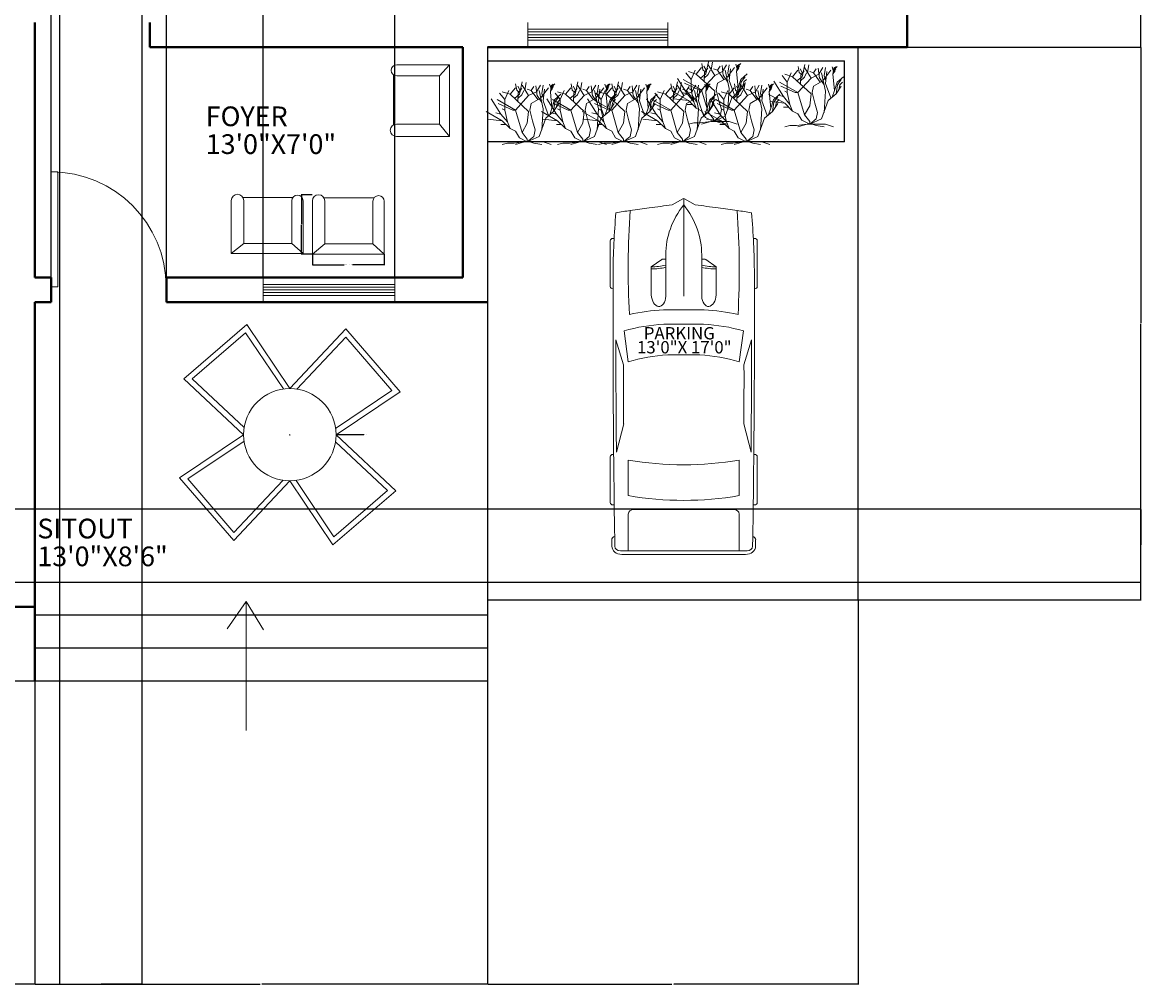
# Model space of a CAD drawing. Units: inches. Extents: x 12978 to 13669, y 46550 to 47327.
# Tile 2 of 5: x 13262 to 13669, y 46550 to 46901. Entities that reach past the tile are written whole.
import ezdxf

# ---------------------------------------------------------------- set-up
doc = ezdxf.new("R2010")
doc.units = ezdxf.units.IN
for name, color, linetype, lineweight in [('A-ANNO-DIMS', 2, 'Continuous', 18), ('A-ANNO-SYMB', 7, 'Continuous', 18), ('A-AREA-IDEN', 1, 'Continuous', 18), ('A-FLOR-OTLN', 7, 'Continuous', 25), ('C-PRKG-VEHI', 8, 'Continuous', 13), ('door', 4, 'Continuous', 20), ('furniture', 5, 'Continuous', 18), ('L-PLNT-TREE', 94, 'Continuous', 13), ('staircase', 7, 'Continuous', 25), ('wall', 7, 'Continuous', 40), ('window', 1, 'Continuous', 18)]:
    doc.layers.add(name, color=color, linetype=linetype, lineweight=lineweight)
doc.styles.get("Standard").update_dxf_attribs({"font": 'arial.ttf'})
doc.dimstyles.get("Standard").update_dxf_attribs({"dimtxt": 0.18, "dimasz": 0.18, "dimexe": 0.18, "dimexo": 0.0625, "dimgap": 0.09, "dimtad": 0, "dimtih": 1, "dimtoh": 1, "dimdec": 4, "dimzin": 0, "dimdsep": 46, "dimtxsty": 'Standard', "dimcen": 0.09, "dimadec": 0, "dimazin": 0, "dimtfac": 1, "dimtdec": 4, "dimtofl": 0, "dimtmove": 0, "dimatfit": 3, "dimfxl": 1, "dimtolj": 1, "dimtzin": 0, "dimarcsym": 0})

# ---------------------------------------------------------------- blocks, each defined once
blk = doc.blocks.new('*U2')
for p, q in [((0, 0), (0, -100)), ((750, 0), (750, -100))]:
    blk.add_line(p, q)
blk.add_lwpolyline([(0, 0), (0, 750), (43.75, 750), (43.75, 0)], close=True)
blk.add_arc((0, 0), 750, 0, 90)
blk = doc.blocks.new('*U6')
at = {"layer": 'furniture'}
for p, q in [((-20.08, -2.46), (0.34, 19.3)), ((0.34, 19.3), (20.08, -3.61)), ((-17.52, -2.66), (0.28, 16.31)), ((0.28, 16.31), (17.1, -3.21)), ((17.1, -3.21), (-3.41, -16.99)), ((20.08, -3.61), (-3.25, -19.3))]:
    blk.add_line(p, q, dxfattribs=at)
blk = doc.blocks.new('*U7')
at = {"layer": 'furniture', "transparency": 16777216}
for p, rotation in [((13339.66, 46770.42), 89.99999999999999), ((13338.88, 46731.04), 180), ((13378.26, 46730.25), 270)]:
    blk.add_blockref('*U6', p, dxfattribs=dict(at, rotation=rotation))
blk.add_blockref('*U6', (13379.05, 46769.63), dxfattribs=at)
blk = doc.blocks.new('*U11')
for p, q in [((21.1, 37.41), (21.1, 36.83)), ((46.55, 38.89), (22.35, 38.89)), ((47.8, 37.39), (47.8, 37.41)), ((87.99, 31.87), (74.76, 35.92)), ((134.31, 35.6), (119.29, 31.78)), ((135.45, 37.07), (135.45, 37.41)), ((136.7, 38.89), (160.9, 38.89)), ((162.15, 37.41), (162.15, 36.77)), ((70.03, 31.54), (86.41, 29.35)), ((186.47, -33.5), (186.47, 33.5)), ((188.4, -32.76), (188.4, 32.76)), ((138.42, 29.35), (157.25, 29.35)), ((164.52, 26.39), (164.52, -26.39)), ((186.47, 29.35), (167.01, 29.35)), ((32.27, 11.63), (36.13, 17.17)), ((36.13, 17.17), (50.94, 17.17)), ((3.27, 6.13), (0.1, 0.41)), ((29.77, 9.51), (51.68, 9.51)), ((32.12, 9.51), (32.12, 11.15)), ((58.92, -10.77), (58.92, 10.77)), ((66.55, -10.53), (66.55, 10.53)), ((82.74, 8.5), (82.74, -8.5)), ((186.47, -10.53), (186.47, 10.53)), ((0, 0), (51.68, 0)), ((0.1, -0.41), (3.27, -6.13)), ((29.77, -9.51), (51.68, -9.51)), ((32.12, -9.51), (32.12, -11.15)), ((32.27, -11.63), (36.13, -17.17)), ((36.13, -17.17), (50.94, -17.17)), ((86.41, -29.35), (70.03, -31.54)), ((157.25, -29.35), (138.42, -29.35)), ((167.01, -29.35), (186.47, -29.35)), ((87.99, -31.87), (74.76, -35.92)), ((134.31, -35.6), (119.29, -31.78)), ((21.1, -37.41), (21.1, -36.83)), ((46.55, -38.89), (22.35, -38.89)), ((47.8, -37.39), (47.8, -37.41)), ((135.45, -37.07), (135.45, -37.41)), ((136.7, -38.89), (160.9, -38.89)), ((162.15, -37.41), (162.15, -36.77))]:
    blk.add_line(p, q)
for centre, major_axis, ratio, start_param, end_param in [((266.03, -27.52), (0, 313.31), 0.842304, 1.367076, 1.39176), ((41.19, -490.86), (0, 528.23), 0.842304, 0.00281, 0.075598), ((22.35, 37.41), (0, -1.48), 0.842304, 3.141593, 4.712389), ((64.48, -10555.62), (0, 10593.03), 0.842304, -0.013397, 0.002797), ((46.55, 37.41), (0, 1.48), 0.842304, -1.570796, 0), ((64.48, -10555.62), (0, -10591.55), 0.842304, 3.133765, 3.140441), ((136.7, 37.41), (0, -1.48), 0.842304, 3.141593, 4.712389), ((160.9, 37.41), (0, 1.48), 0.842304, -1.570796, 0), ((180.63, 35.84), (0, 2.22), 0.842304, -0.013017, 1.249894), ((64.48, -10556.36), (0, 10595.31), 0.842304, -0.013397, -0.013017), ((183.98, 33.5), (0, -2.96), 0.842304, 1.570796, 3.128196), ((183.98, 32.76), (0, -5.25), 0.842304, 1.570796, 3.128196), ((37.47, -593.96), (0, -623.33), 0.842304, 3.096046, 3.200911), ((135.29, 5.39), (0, 81.77), 0.842304, 1.245306, 1.50788), ((95.79, -3666.35), (0, -3698.24), 0.842304, 3.134049, 3.144098), ((259.18, -27.52), (0, -305.3), 0.842304, 4.528606, 4.561838), ((134.4, 5.39), (0, -89.78), 0.842304, 4.449482, 4.652344), ((149.6, 2.8), (0, -79.58), 0.842304, 4.372215, 4.640744), ((17.08, 0), (0, 147.02), 0.842304, 4.511394, 4.913384), ((35.91, 0), (0, 147.02), 0.842304, 4.511394, 4.913384), ((167.01, 26.39), (0, 2.96), 0.842304, 0, 1.570796), ((-204.49, 52.4), (0, -250.96), 0.842304, 1.385369, 1.434372), ((13.04, 17.01), (0, 27.42), 0.842304, 4.435146, 4.718221), ((14.2, 17.01), (0, 27.42), 0.842304, 4.435146, 4.718221), ((50.79, 13.34), (6.34, -0.36), 0.603834, -1.395552, 1.581315), ((29.77, -46.66), (0, 56.17), 0.842304, 0, 0.590319), ((32.75, 11.15), (0, 0.74), 0.842304, 0.879714, 1.570796), ((0.62, 0), (0, -0.74), 0.842304, 4.131459, 5.293319), ((29.77, 46.66), (0, 56.17), 0.842304, 2.551274, 3.141593), ((-204.49, -52.4), (0, 250.96), 0.842304, -1.434372, -1.385369), ((32.75, -11.15), (0, -0.74), 0.842304, 4.712389, 5.403472), ((13.04, -17.01), (0, -27.42), 0.842304, 1.564964, 1.848039), ((14.2, -17.01), (0, -27.42), 0.842304, 1.564964, 1.848039), ((134.4, -5.39), (0, -89.78), 0.842304, -1.510751, -1.307889), ((135.29, -5.39), (0, -81.77), 0.842304, -1.50788, -1.245306), ((149.6, -2.8), (0, -79.58), 0.842304, -1.499151, -1.230623), ((259.18, 27.52), (0, 305.3), 0.842304, 1.721348, 1.754579), ((266.03, 27.52), (0, 313.31), 0.842304, 1.749832, 1.774517), ((37.47, 593.96), (0, -623.33), 0.842304, -0.059319, 0.045547), ((167.01, -26.39), (0, -2.96), 0.842304, 4.712389, 6.283185), ((95.79, 3666.35), (0, -3698.24), 0.842304, -0.002505, 0.007544), ((183.98, -33.5), (0, 2.96), 0.842304, 3.15499, 4.712389), ((183.98, -32.76), (0, -5.25), 0.842304, 0.013397, 1.570796), ((41.19, 490.86), (0, -528.23), 0.842304, -0.075598, -0.00281), ((22.35, -37.41), (0, 1.48), 0.842304, 1.570796, 3.141593), ((64.48, 10555.62), (0, 10593.03), 0.842304, 3.138796, 3.15499), ((46.55, -37.41), (0, -1.48), 0.842304, 0, 1.570796), ((64.48, 10555.62), (0, -10591.55), 0.842304, 0.001152, 0.007828), ((136.7, -37.41), (0, -1.48), 0.842304, -1.570796, 0), ((160.9, -37.41), (0, 1.48), 0.842304, 3.141593, 4.712389), ((180.63, -35.84), (0, -2.22), 0.842304, -1.249894, 0.013017), ((64.48, 10556.36), (0, 10595.31), 0.842304, 3.15461, 3.15499)]:
    blk.add_ellipse(centre, major_axis=major_axis, ratio=ratio, start_param=start_param, end_param=end_param)
at = {"extrusion": (0, 0, -1)}
blk.add_ellipse((50.79, -13.34), major_axis=(6.34, 0.36), ratio=0.603834, start_param=-1.395552, end_param=1.581315, dxfattribs=at)
blk = doc.blocks.new('*U13')
for p, q in [((-14.88, 18.24), (-12.96, 20.64)), ((-12.471, 19.775), (-12.898, 22.044)), ((-11.28, 19.619), (-12.104, 21.184)), ((-11.921, 18.836), (-10.64, 20.401)), ((-11.433, 18.289), (-10.457, 22.749)), ((-8.16, 17.76), (-10.56, 21.6)), ((-9.48, 19.775), (-8.992, 22.592)), ((-7.2, 19.68), (-6.24, 21.12)), ((-5.086, 17.741), (-5.513, 21.34)), ((-5.28, 19.2), (-3.84, 21.6)), ((-3.84, 16.8), (-0.96, 20.64)), ((-3.377, 18.602), (-2.888, 21.575)), ((-0.508, 21.888), (-0.081, 20.558)), ((-0.203, 19.149), (0.102, 21.34)), ((-0.142, 19.384), (0.59, 20.401)), ((-0.02, 20.01), (0.896, 21.105)), ((0.041, 20.714), (1.384, 22.044)), ((0.102, 21.34), (0.835, 21.888)), ((-18.24, 11.04), (-21.755, 16.655)), ((-12.96, 12.48), (-19.68, 16.32)), ((-16.8, 16.32), (-18.72, 18.72)), ((-14.88, 18.24), (-17.76, 19.2)), ((-16.8, 16.32), (-15.36, 19.68)), ((-16.8, 12.48), (-16.8, 16.32)), ((-8.16, 12), (-14.88, 18.24)), ((-13.325, 16.724), (-11.433, 18.289)), ((-12.96, 12.48), (-8.16, 17.76)), ((-11.677, 19.071), (-12.471, 19.775)), ((-12.043, 15.628), (-11.921, 18.836)), ((-11.982, 16.802), (-10.579, 18.054)), ((-10.579, 18.054), (-9.846, 19.697)), ((-7.2, 19.68), (-8.64, 20.16)), ((-8.16, 17.76), (-5.28, 19.2)), ((-4.8, 16.32), (-7.2, 19.68)), ((-7.2, 14.88), (-3.84, 16.8)), ((-3.377, 15.315), (-5.086, 17.819)), ((-2.88, 12.96), (-4.32, 19.68)), ((-2.766, 16.802), (-3.377, 18.602)), ((-2.88, 15.84), (-2.4, 20.16)), ((0.346, 13.203), (-0.203, 19.149)), ((1.323, 16.254), (3.642, 18.289)), ((1.44, 15.36), (2.88, 17.28)), ((2.4, 15.36), (3.36, 16.32)), ((-13.92, 12.48), (-19.2, 14.88)), ((-16.8, 12.48), (-17.76, 12.96)), ((-15.84, 8.16), (-16.8, 12.48)), ((-12.96, 12.48), (-13.92, 12.48)), ((-10.56, 4.32), (-12.96, 12.48)), ((-7.68, 12.48), (-7.2, 14.88)), ((-6.72, 8.64), (-7.68, 12.48)), ((-3.36, 5.28), (-2.88, 12.96)), ((-0.96, 10.56), (-2.88, 15.84)), ((-0.48, 10.8), (0.346, 13.203)), ((0.346, 13.203), (1.323, 16.254)), ((0.96, 12), (1.44, 15.36)), ((0.96, 12), (2.88, 14.88)), ((1.92, 13.44), (2.4, 15.36)), ((-17.76, 8.64), (-23.663, 11.961)), ((-17.76, 8.64), (-23.128, 9.222)), ((-18.24, 11.04), (-20.16, 11.52)), ((-15.84, 8.16), (-18.24, 11.04)), ((-14.88, 5.76), (-17.76, 8.64)), ((-14.88, 5.76), (-15.84, 8.16)), ((-8.64, 7.68), (-8.16, 12)), ((-5.76, 5.28), (-6.72, 8.64)), ((-4.32, 2.88), (-1.92, 9.6)), ((-1.92, 9.6), (0.96, 12)), ((-16.32, 7.2), (-18.24, 7.2)), ((-12.96, 4.8), (-14.88, 5.76)), ((-11.52, 2.4), (-12.96, 4.8)), ((-10.56, 4.32), (-8.64, 7.68)), ((-8.64, 1.92), (-10.56, 4.32)), ((-6.24, 2.88), (-5.76, 5.28)), ((-15.84, 0.48), (-17.76, 0)), ((-13.44, 0.48), (-15.84, 0.48)), ((-9.6, 0.96), (-13.44, 0.48)), ((-9.6, 0.96), (-12.96, 0)), ((-8.64, 0.96), (-11.52, 2.4)), ((-9.6, 0.96), (-7.68, 0.96)), ((-8.64, 0.96), (-4.32, 2.88)), ((-8.64, 0.96), (-6.24, 2.88)), ((-8.64, 0.96), (-8.64, 1.92)), ((-8.64, 0.96), (-2.88, 0.96)), ((-7.68, 0.96), (-6.24, 0.48)), ((-6.24, 0.48), (-3.36, 0)), ((-2.88, 0.96), (0, 0))]:
    blk.add_line(p, q)
blk = doc.blocks.new('WINDOW-51')
for p, q in [((0, 0), (0, 9)), ((51.08, 0), (51.08, 9)), ((0, 6.5), (51.08, 6.5)), ((0, 5.5), (51.08, 5.5)), ((0, 4.5), (51.08, 4.5)), ((0, 3.5), (51.08, 3.5)), ((0, 2.5), (51.08, 2.5))]:
    blk.add_line(p, q)
blk = doc.blocks.new('CHAIR-LOUNGE')
for p, q in [((21.6, 26.17), (2.34, 26.17)), ((17.92, 22.06), (21.6, 26.17)), ((21.6, 0), (21.6, 26.17)), ((1.14, 4.21), (1.14, 22.45)), ((2.34, 22.06), (17.92, 22.06)), ((17.92, 22.06), (17.92, 4.51)), ((17.92, 4.51), (2.25, 4.51)), ((17.92, 4.51), (21.6, 0)), ((2.25, 0), (21.6, 0))]:
    blk.add_line(p, q)
for centre, radius in [((2.34, 24.11), 2.05), ((2.25, 2.25), 2.25)]:
    blk.add_arc(centre, radius, 90, 270)
blk = doc.blocks.new('*D41')
at = {"layer": 'A-ANNO-DIMS', "color": 0, "lineweight": -2, "transparency": 16777216}
for p, q in [((13367.21, 46816.14), (13367.21, 46812.09)), ((13393.37, 46816.14), (13393.37, 46812.09)), ((13367.39, 46812.27), (13378.78, 46812.27)), ((13393.19, 46812.27), (13381.81, 46812.27))]:
    blk.add_line(p, q, dxfattribs=at)
at = {"layer": 'A-ANNO-DIMS', "color": 0, "transparency": 16777216}
for points in [[(13367.39, 46812.3), (13367.39, 46812.24), (13367.21, 46812.27)], [(13393.19, 46812.3), (13393.19, 46812.24), (13393.37, 46812.27)]]:
    blk.add_solid(points, dxfattribs=at)
at = {"layer": 'Defpoints', "color": 0, "transparency": 16777216}
for p in [(13367.21, 46816.2), (13393.37, 46816.2), (13393.37, 46812.27)]:
    blk.add_point(p, dxfattribs=at)
at = {"layer": 'A-ANNO-DIMS', "color": 0, "transparency": 16777216, "insert": (13380.29, 46812.27), "char_height": 0.18, "attachment_point": 5}
blk.add_mtext('\\A1;LOUNGE CHAIR 26 TYP.', dxfattribs=at)
blk = doc.blocks.new('*D42')
at = {"layer": 'A-ANNO-DIMS', "color": 0, "lineweight": -2, "transparency": 16777216}
for p, q in [((13367.15, 46837.79), (13363.1, 46837.79)), ((13363.28, 46837.61), (13363.28, 46827.18)), ((13363.28, 46816.38), (13363.28, 46826.82)), ((13367.15, 46816.2), (13363.1, 46816.2))]:
    blk.add_line(p, q, dxfattribs=at)
at = {"layer": 'A-ANNO-DIMS', "color": 0, "transparency": 16777216}
for points in [[(13363.25, 46837.61), (13363.31, 46837.61), (13363.28, 46837.79)], [(13363.25, 46816.38), (13363.31, 46816.38), (13363.28, 46816.2)]]:
    blk.add_solid(points, dxfattribs=at)
at = {"layer": 'Defpoints', "color": 0, "transparency": 16777216}
for p in [(13367.21, 46837.79), (13363.28, 46816.2), (13367.21, 46816.2)]:
    blk.add_point(p, dxfattribs=at)
at = {"layer": 'A-ANNO-DIMS', "color": 0, "transparency": 16777216, "insert": (13363.28, 46827), "char_height": 0.18, "attachment_point": 5}
blk.add_mtext('\\A1;22 TYP.', dxfattribs=at)
blk = doc.blocks.new('*D57')
at = {"layer": 'A-ANNO-DIMS', "color": 0, "lineweight": -2, "transparency": 16777216}
for p, q in [((13575.07, 47080.63), (13669.26, 47080.63)), ((13669.08, 47080.45), (13669.08, 46986.32)), ((13669.08, 46891.81), (13669.08, 46985.95)), ((13584.07, 46891.63), (13669.26, 46891.63))]:
    blk.add_line(p, q, dxfattribs=at)
at = {"layer": 'A-ANNO-DIMS', "color": 0, "transparency": 16777216}
for points in [[(13669.05, 47080.45), (13669.11, 47080.45), (13669.08, 47080.63)], [(13669.05, 46891.81), (13669.11, 46891.81), (13669.08, 46891.63)]]:
    blk.add_solid(points, dxfattribs=at)
at = {"layer": 'Defpoints', "color": 0, "transparency": 16777216}
for p in [(13575.01, 47080.63), (13669.08, 47080.63), (13584.01, 46891.63)]:
    blk.add_point(p, dxfattribs=at)
at = {"layer": 'A-ANNO-DIMS', "color": 0, "transparency": 16777216, "insert": (13669.08, 46986.13), "char_height": 0.18, "attachment_point": 5}
blk.add_mtext('\\A1;189', dxfattribs=at)
blk = doc.blocks.new('*D59')
at = {"layer": 'A-ANNO-DIMS', "color": 0, "lineweight": -2, "transparency": 16777216}
for p, q in [((13566.15, 46891.63), (13669.26, 46891.63)), ((13669.08, 46891.45), (13669.08, 46791.06)), ((13669.08, 46690.31), (13669.08, 46790.7)), ((13566.15, 46690.13), (13669.26, 46690.13))]:
    blk.add_line(p, q, dxfattribs=at)
at = {"layer": 'A-ANNO-DIMS', "color": 0, "transparency": 16777216}
for points in [[(13669.05, 46891.45), (13669.11, 46891.45), (13669.08, 46891.63)], [(13669.05, 46690.31), (13669.11, 46690.31), (13669.08, 46690.13)]]:
    blk.add_solid(points, dxfattribs=at)
at = {"layer": 'Defpoints', "color": 0, "transparency": 16777216}
for p in [(13566.09, 46891.63), (13669.08, 46891.63), (13566.09, 46690.13)]:
    blk.add_point(p, dxfattribs=at)
at = {"layer": 'A-ANNO-DIMS', "color": 0, "transparency": 16777216, "insert": (13669.08, 46790.88), "char_height": 0.18, "attachment_point": 5}
blk.add_mtext('\\A1;201.5', dxfattribs=at)
blk = doc.blocks.new('*D60')
at = {"layer": 'A-ANNO-DIMS', "color": 0, "lineweight": -2, "transparency": 16777216}
for p, q in [((13059.005025, 46660.571951), (13059.005025, 46549.877451)), ((13266.005025, 46660.571951), (13266.005025, 46549.877451)), ((13059.185025, 46550.057451), (13162.214643, 46550.057451)), ((13265.825025, 46550.057451), (13162.795407, 46550.057451))]:
    blk.add_line(p, q, dxfattribs=at)
at = {"layer": 'A-ANNO-DIMS', "color": 0, "transparency": 16777216}
for points in [[(13059.185025, 46550.087451), (13059.185025, 46550.027451), (13059.005025, 46550.057451)], [(13265.825025, 46550.087451), (13265.825025, 46550.027451), (13266.005025, 46550.057451)]]:
    blk.add_solid(points, dxfattribs=at)
at = {"layer": 'Defpoints', "color": 0, "transparency": 16777216}
for p in [(13059.005025, 46660.634451), (13266.005025, 46660.634451), (13266.005025, 46550.057451)]:
    blk.add_point(p, dxfattribs=at)
at = {"layer": 'A-ANNO-DIMS', "color": 0, "transparency": 16777216, "insert": (13162.505025, 46550.057451), "char_height": 0.18, "attachment_point": 5}
blk.add_mtext('\\A1;207', dxfattribs=at)
blk = doc.blocks.new('*D61')
at = {"layer": 'A-ANNO-DIMS', "color": 0, "lineweight": -2, "transparency": 16777216}
for p, q in [((13266.01, 46660.57), (13266.01, 46549.88)), ((13431.01, 46660.57), (13431.01, 46549.88)), ((13266.19, 46550.06), (13348.22, 46550.06)), ((13430.83, 46550.06), (13348.79, 46550.06))]:
    blk.add_line(p, q, dxfattribs=at)
at = {"layer": 'A-ANNO-DIMS', "color": 0, "transparency": 16777216}
for points in [[(13266.19, 46550.09), (13266.19, 46550.03), (13266.01, 46550.06)], [(13430.83, 46550.09), (13430.83, 46550.03), (13431.01, 46550.06)]]:
    blk.add_solid(points, dxfattribs=at)
at = {"layer": 'Defpoints', "color": 0, "transparency": 16777216}
for p in [(13266.01, 46660.63), (13431.01, 46660.63), (13431.01, 46550.06)]:
    blk.add_point(p, dxfattribs=at)
at = {"layer": 'A-ANNO-DIMS', "color": 0, "transparency": 16777216, "insert": (13348.51, 46550.06), "char_height": 0.18, "attachment_point": 5}
blk.add_mtext('\\A1;165', dxfattribs=at)
blk = doc.blocks.new('*D62')
at = {"layer": 'A-ANNO-DIMS', "color": 0, "lineweight": -2, "transparency": 16777216}
for p, q in [((13431.01, 46690.07), (13431.01, 46549.88)), ((13566.09, 46690.07), (13566.09, 46549.88)), ((13431.19, 46550.06), (13498.18, 46550.06)), ((13565.91, 46550.06), (13498.92, 46550.06))]:
    blk.add_line(p, q, dxfattribs=at)
at = {"layer": 'A-ANNO-DIMS', "color": 0, "transparency": 16777216}
for points in [[(13431.19, 46550.09), (13431.19, 46550.03), (13431.01, 46550.06)], [(13565.91, 46550.09), (13565.91, 46550.03), (13566.09, 46550.06)]]:
    blk.add_solid(points, dxfattribs=at)
at = {"layer": 'Defpoints', "color": 0, "transparency": 16777216}
for p in [(13431.01, 46690.13), (13566.09, 46690.13), (13566.09, 46550.06)]:
    blk.add_point(p, dxfattribs=at)
at = {"layer": 'A-ANNO-DIMS', "color": 0, "transparency": 16777216, "insert": (13498.55, 46550.06), "char_height": 0.18, "attachment_point": 5}
blk.add_mtext('\\A1;135.1', dxfattribs=at)
blk = doc.blocks.new('*D63')
at = {"layer": 'A-ANNO-DIMS', "color": 0, "lineweight": -2, "transparency": 16777216}
for p, q in [((13275.01, 47169.07), (13275.01, 46549.88)), ((13305.01, 47169.07), (13305.01, 46549.88)), ((13275.19, 46550.06), (13289.79, 46550.06)), ((13304.83, 46550.06), (13290.22, 46550.06))]:
    blk.add_line(p, q, dxfattribs=at)
at = {"layer": 'A-ANNO-DIMS', "color": 0, "transparency": 16777216}
for points in [[(13275.19, 46550.09), (13275.19, 46550.03), (13275.01, 46550.06)], [(13304.83, 46550.09), (13304.83, 46550.03), (13305.01, 46550.06)]]:
    blk.add_solid(points, dxfattribs=at)
at = {"layer": 'Defpoints', "color": 0, "transparency": 16777216}
for p in [(13275.01, 47169.13), (13305.01, 47169.13), (13305.01, 46550.06)]:
    blk.add_point(p, dxfattribs=at)
at = {"layer": 'A-ANNO-DIMS', "color": 0, "transparency": 16777216, "insert": (13290.01, 46550.06), "char_height": 0.18, "attachment_point": 5}
blk.add_mtext('\\A1;30', dxfattribs=at)
blk = doc.blocks.new('*D64')
at = {"layer": 'A-ANNO-DIMS', "color": 0, "lineweight": -2, "transparency": 16777216}
for p, q in [((13272.01, 46807.7), (13272.01, 47304.06)), ((13272.19, 47303.88), (13292.78, 47303.88)), ((13313.83, 47303.88), (13293.23, 47303.88)), ((13314.01, 46807.7), (13314.01, 47304.06))]:
    blk.add_line(p, q, dxfattribs=at)
at = {"layer": 'A-ANNO-DIMS', "color": 0, "transparency": 16777216}
for points in [[(13272.19, 47303.91), (13272.19, 47303.85), (13272.01, 47303.88)], [(13313.83, 47303.91), (13313.83, 47303.85), (13314.01, 47303.88)]]:
    blk.add_solid(points, dxfattribs=at)
at = {"layer": 'Defpoints', "color": 0, "transparency": 16777216}
for p in [(13314.01, 47303.88), (13272.01, 46807.63), (13314.01, 46807.63)]:
    blk.add_point(p, dxfattribs=at)
at = {"layer": 'A-ANNO-DIMS', "color": 0, "transparency": 16777216, "insert": (13293.01, 47303.88), "char_height": 0.18, "attachment_point": 5}
blk.add_mtext('\\A1;42', dxfattribs=at)
blk = doc.blocks.new('*D65')
at = {"layer": 'A-ANNO-DIMS', "color": 0, "lineweight": -2, "transparency": 16777216}
for p, q in [((13349.22, 46807.7), (13349.22, 47304.06)), ((13349.4, 47303.88), (13373, 47303.88)), ((13397.04, 47303.88), (13373.45, 47303.88)), ((13397.22, 46807.7), (13397.22, 47304.06))]:
    blk.add_line(p, q, dxfattribs=at)
at = {"layer": 'A-ANNO-DIMS', "color": 0, "transparency": 16777216}
for points in [[(13349.4, 47303.91), (13349.4, 47303.85), (13349.22, 47303.88)], [(13397.04, 47303.91), (13397.04, 47303.85), (13397.22, 47303.88)]]:
    blk.add_solid(points, dxfattribs=at)
at = {"layer": 'Defpoints', "color": 0, "transparency": 16777216}
for p in [(13397.22, 47303.88), (13349.22, 46807.63), (13397.22, 46807.63)]:
    blk.add_point(p, dxfattribs=at)
at = {"layer": 'A-ANNO-DIMS', "color": 0, "transparency": 16777216, "insert": (13373.22, 47303.88), "char_height": 0.18, "attachment_point": 5}
blk.add_mtext('\\A1;48', dxfattribs=at)
blk = doc.blocks.new('*D78')
at = {"layer": 'A-ANNO-DIMS', "color": 0, "lineweight": -2, "transparency": 16777216}
for p, q in [((13224.37, 46723.29), (13669.26, 46723.29)), ((13669.08, 46723.11), (13669.08, 46710.15)), ((13669.08, 46696.81), (13669.08, 46709.78)), ((13257.07, 46696.63), (13669.26, 46696.63))]:
    blk.add_line(p, q, dxfattribs=at)
at = {"layer": 'A-ANNO-DIMS', "color": 0, "transparency": 16777216}
for points in [[(13669.05, 46723.11), (13669.11, 46723.11), (13669.08, 46723.29)], [(13669.05, 46696.81), (13669.11, 46696.81), (13669.08, 46696.63)]]:
    blk.add_solid(points, dxfattribs=at)
at = {"layer": 'Defpoints', "color": 0, "transparency": 16777216}
for p in [(13224.3, 46723.29), (13669.08, 46723.29), (13257.01, 46696.63)]:
    blk.add_point(p, dxfattribs=at)
at = {"layer": 'A-ANNO-DIMS', "color": 0, "transparency": 16777216, "insert": (13669.08, 46709.96), "char_height": 0.18, "attachment_point": 5}
blk.add_mtext('\\A1;26.66', dxfattribs=at)
blk = doc.blocks.new('*D79')
at = {"layer": 'A-ANNO-DIMS', "color": 0, "lineweight": -2, "transparency": 16777216}
for p, q in [((13358.87, 46750.33), (13359.05, 46750.33)), ((13358.96, 46750.24), (13358.96, 46750.42)), ((13385.9, 46750.34), (13375.98, 46750.33))]:
    blk.add_line(p, q, dxfattribs=at)
at = {"layer": 'A-ANNO-DIMS', "color": 0, "transparency": 16777216}
blk.add_solid([(13375.98, 46750.37), (13375.98, 46750.31), (13375.8, 46750.33)], dxfattribs=at)
at = {"layer": 'Defpoints', "color": 0, "transparency": 16777216}
for p in [(13342.13, 46750.33), (13375.8, 46750.33)]:
    blk.add_point(p, dxfattribs=at)
at = {"layer": 'A-ANNO-DIMS', "color": 0, "transparency": 16777216, "insert": (13386.39, 46750.34), "char_height": 0.18, "attachment_point": 5}
blk.add_mtext('\\A1;∅33.67', dxfattribs=at)

msp = doc.modelspace()

# ---------------------------------------------------------------- linework, layer by layer
at = {"layer": 'A-ANNO-SYMB'}
for p, q in [((13343.0969, 46689.5271), (13336.0741, 46679.6103)), ((13343.0969, 46642.5353), (13343.0969, 46689.5271)), ((13343.0969, 46689.5271), (13349.3877, 46679.2043))]:
    msp.add_line(p, q, dxfattribs=at)
at = {"layer": 'A-FLOR-OTLN'}
for p, q in [((13431.005, 46891.6345), (13431.005, 46660.6345)), ((13566.0922, 46857.1263), (13566.0922, 46891.6345)), ((13431.005, 46886.6345), (13561.0922, 46886.6345)), ((13561.0922, 46857.1263), (13561.0922, 46886.6345)), ((13059.005, 46660.6345), (13431.005, 46660.6345))]:
    msp.add_line(p, q, dxfattribs=at)
msp.add_lwpolyline([(13561.0922, 46857.1263), (13431.005, 46857.1263), (13431.005, 46690.1305), (13566.0922, 46690.1305), (13566.0922, 46857.1263)], dxfattribs=at)
at = {"layer": 'furniture'}
msp.add_circle((13358.9612, 46750.3348), 16.8359, dxfattribs=at)
at = {"layer": 'staircase'}
for p, q in [((13266.005, 46696.6345), (13431.005, 46696.6345)), ((13266.005, 46684.6345), (13431.005, 46684.6345)), ((13266.005, 46672.6345), (13431.005, 46672.6345))]:
    msp.add_line(p, q, dxfattribs=at)
at = {"layer": 'wall'}
for p, q in [((13584.005, 47266.6345), (13584.005, 46891.6345)), ((13266.005, 46900.6345), (13266.005, 46807.6345)), ((13308.005, 46900.6345), (13308.005, 46891.6345)), ((13308.005, 46891.6345), (13422.005, 46891.6345)), ((13422.005, 46891.6345), (13422.005, 46807.6345)), ((13431.005, 46891.6345), (13584.005, 46891.6345)), ((13266.005, 46807.6345), (13272.005, 46807.6345)), ((13272.005, 46807.6345), (13272.005, 46798.6345)), ((13314.005, 46807.6345), (13314.005, 46798.6345)), ((13314.005, 46807.6345), (13422.005, 46807.6345)), ((13266.005, 46798.6345), (13272.005, 46798.6345)), ((13266.005, 46798.6345), (13266.005, 46660.6345)), ((13314.005, 46798.6345), (13431.005, 46798.6345)), ((13059.005, 46687.6345), (13266.005, 46687.6345))]:
    msp.add_line(p, q, dxfattribs=at)
at = {"layer": 'window'}
for p, q in [((13349.2243, 46798.6345), (13349.2243, 46807.6345)), ((13349.2243, 46805.1345), (13397.2243, 46805.1345)), ((13397.2243, 46798.6345), (13397.2243, 46807.6345)), ((13349.2243, 46804.1345), (13397.2243, 46804.1345)), ((13349.2243, 46803.1345), (13397.2243, 46803.1345)), ((13349.2243, 46802.1345), (13397.2243, 46802.1345)), ((13349.2243, 46801.1345), (13397.2243, 46801.1345))]:
    msp.add_line(p, q, dxfattribs=at)

# ---------------------------------------------------------------- block references
at = {"layer": 'C-PRKG-VEHI', "xscale": 0.6887919479552651, "yscale": 0.6887919479552651, "zscale": 0.6887919479552651, "rotation": 270}
msp.add_blockref('*U11', (13502.5212, 46836.4367), dxfattribs=at)
at = {"layer": 'door', "xscale": 0.0558759688399716, "yscale": 0.0558759688399716, "zscale": 0.0558759688399716}
msp.add_blockref('*U2', (13272.005, 46804.222), dxfattribs=at)
at = {"layer": 'furniture'}
for name, p in [('CHAIR-LOUNGE', (13395.5871, 46859.0438)), ('*U7', (0, 0))]:
    msp.add_blockref(name, p, dxfattribs=at)
for p, rotation in [((13337.649, 46837.9701), 269.9999999999682), ((13367.208, 46837.7944), 269.9999999999491)]:
    msp.add_blockref('CHAIR-LOUNGE', p, dxfattribs=dict(at, rotation=rotation))
at = {"layer": 'L-PLNT-TREE'}
for p in [(13521.9866, 46863.5477), (13557.0633, 46862.5561), (13454.1498, 46856.1663), (13474.3353, 46856.1663), (13489.2265, 46856.1663), (13510.7357, 46856.1663), (13533.8995, 46856.1663)]:
    msp.add_blockref('*U13', p, dxfattribs=at)
at = {"layer": 'window', "rotation": 180}
msp.add_blockref('WINDOW-51', (13496.7677, 46900.6345), dxfattribs=at)

# ---------------------------------------------------------------- texts
at = {"layer": 'A-AREA-IDEN'}
for s, height, p in [('FOYER', 7.17855, (13328.3234, 46862.7983)), ('13\'0"X7\'0"', 7.17855, (13328.3234, 46852.6598)), ('PARKING', 4.48664, (13487.9632, 46785.0702)), ('13\'0"X 17\'0"', 4.486642, (13485.5033, 46779.9674)), ('SITOUT', 7.17855, (13266.955, 46712.5365)), ('13\'0"X8\'6"', 7.17855, (13266.955, 46702.398))]:
    msp.add_text(s, height=height, dxfattribs=at).set_placement(p)

# ---------------------------------------------------------------- dimensions: what is measured, and where the dimension line sits
at = {"layer": 'A-ANNO-DIMS'}
for base, p1, p2, override, picture, middle in [((13314.005, 47303.8845), (13272.005, 46807.6345), (13314.005, 46807.6345), {"dimdec": 0, "dimlfac": 1, "dimrnd": 0, "dimzin": 0, "dimdsep": 46, "dimlunit": 2}, '*D64', (13293.005, 47303.8845)), ((13397.2243, 47303.8845), (13349.2243, 46807.6345), (13397.2243, 46807.6345), {"dimdec": 0, "dimlfac": 1, "dimrnd": 0, "dimzin": 0, "dimdsep": 46, "dimlunit": 2}, '*D65', (13373.2243, 47303.8845)), ((13305.005, 46550.0575), (13275.005, 47169.1345), (13305.005, 47169.1345), {"dimdec": 0, "dimlfac": 1, "dimrnd": 0, "dimzin": 0, "dimdsep": 46, "dimlunit": 2}, '*D63', (13290.005, 46550.0575)), ((13566.0922, 46550.0575), (13431.005, 46690.1305), (13566.0922, 46690.1305), {"dimdec": 1, "dimlfac": 1, "dimrnd": 0, "dimzin": 0, "dimdsep": 46, "dimlunit": 2}, '*D62', (13498.5486, 46550.0575)), ((13266.005, 46550.0575), (13059.005, 46660.6345), (13266.005, 46660.6345), {"dimdec": 0, "dimlfac": 1, "dimrnd": 0, "dimzin": 0, "dimdsep": 46, "dimlunit": 2}, '*D60', (13162.505, 46550.0575)), ((13431.005, 46550.0575), (13266.005, 46660.6345), (13431.005, 46660.6345), {"dimdec": 0, "dimlfac": 1, "dimrnd": 0, "dimzin": 0, "dimdsep": 46, "dimlunit": 2}, '*D61', (13348.505, 46550.0575))]:
    dim = msp.add_linear_dim(base=base, p1=p1, p2=p2, dimstyle='Standard', override=override, dxfattribs=at)
    dim.commit()
    dim.dimension.update_dxf_attribs({"geometry": picture, "text_midpoint": middle})
for base, p1, p2, override, picture, middle in [((13669.0793, 47080.6345), (13584.005, 46891.6345), (13575.005, 47080.6345), {"dimdec": 0, "dimlfac": 1, "dimrnd": 0, "dimzin": 0, "dimdsep": 46, "dimlunit": 2}, '*D57', (13669.0793, 46986.1345)), ((13669.0793, 46891.6345), (13566.0922, 46690.1305), (13566.0922, 46891.6345), {"dimdec": 1, "dimlfac": 1, "dimrnd": 0, "dimzin": 0, "dimdsep": 46, "dimlunit": 2}, '*D59', (13669.0793, 46790.8825)), ((13669.0793, 46723.2923), (13257.005, 46696.6345), (13224.303, 46723.2923), {"dimdec": 2, "dimlfac": 1, "dimrnd": 0, "dimzin": 0, "dimdsep": 46, "dimlunit": 2}, '*D78', (13669.0793, 46709.9634))]:
    dim = msp.add_linear_dim(base=base, p1=p1, p2=p2, angle=90, dimstyle='Standard', override=override, dxfattribs=at)
    dim.commit()
    dim.dimension.update_dxf_attribs({"geometry": picture, "text_midpoint": middle})
dim = msp.add_linear_dim(base=(13363.2831, 46816.1977), p1=(13367.208, 46837.7944), p2=(13367.208, 46816.1977), angle=270, text='<> TYP.', dimstyle='Standard', override={"dimdec": 0, "dimlfac": 1, "dimrnd": 0, "dimzin": 0, "dimdsep": 46, "dimlunit": 2}, dxfattribs=at)
dim.commit()
dim.dimension.update_dxf_attribs({"geometry": '*D42', "text_midpoint": (13363.2831, 46826.996)})
dim = msp.add_linear_dim(base=(13393.3743, 46812.2727), p1=(13367.208, 46816.1977), p2=(13393.3743, 46816.1977), text='LOUNGE CHAIR <> TYP.', dimstyle='Standard', override={"dimdec": 0, "dimlfac": 1, "dimrnd": 0, "dimzin": 0, "dimdsep": 46, "dimlunit": 2}, dxfattribs=at)
dim.commit()
dim.dimension.update_dxf_attribs({"geometry": '*D41', "text_midpoint": (13380.2912, 46812.2727)})
dim = msp.add_diameter_dim_2p(p1=(13342.1253, 46750.3346), p2=(13375.7972, 46750.335), dimstyle='Standard', override={"dimdec": 2, "dimlfac": 1, "dimrnd": 0, "dimzin": 0, "dimdsep": 46, "dimlunit": 2}, dxfattribs=at)
dim.commit()
dim.dimension.update_dxf_attribs({"geometry": '*D79', "text_midpoint": (13385.8987, 46750.3351), "dimtype": 163})

doc.saveas('drawing.dxf')
